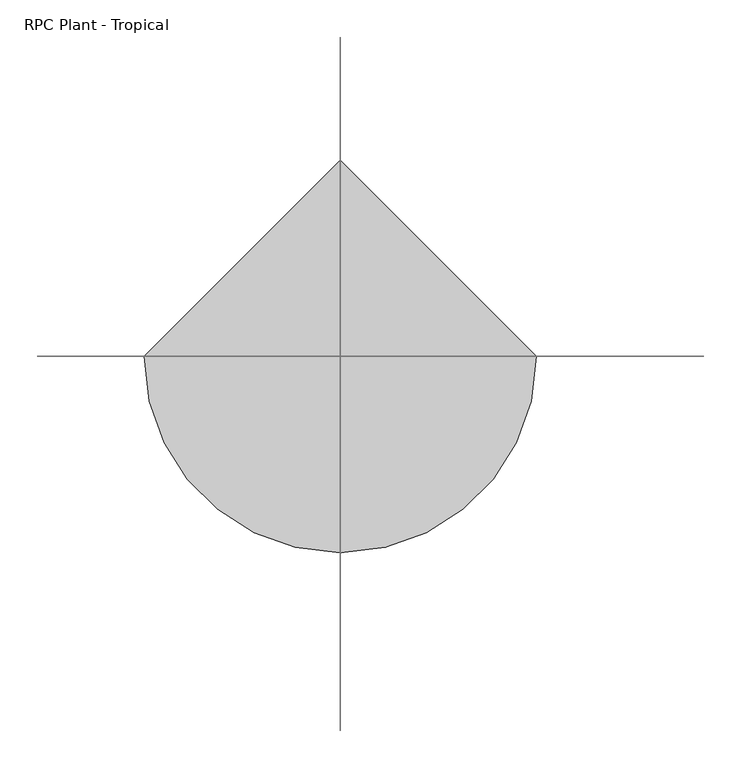
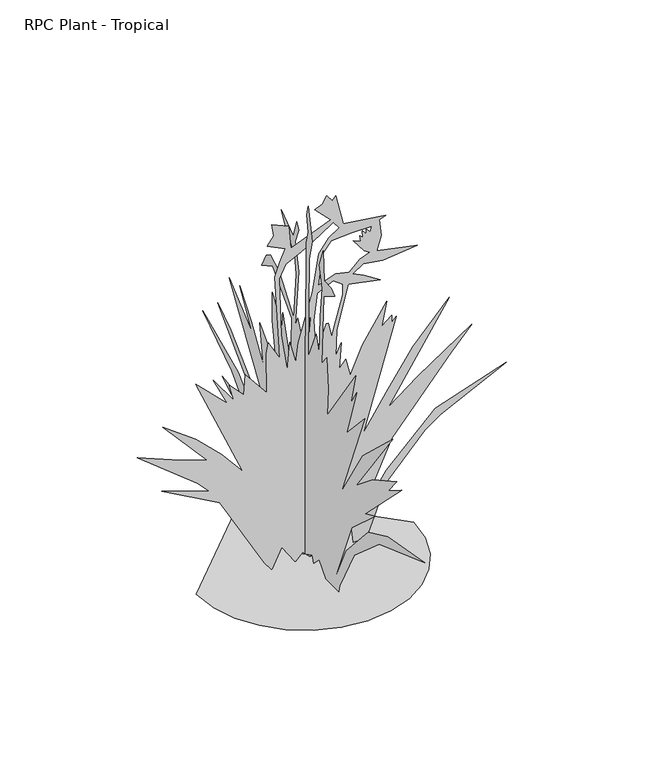
"""IFC4 building model written with IfcOpenShell, lengths in millimetres: geographic element geometry, RPC Plant - Tropical."""

from ifc_helpers import new_model, si_unit, origin, place, context, project, spatial, triangles, source, transform, mapped, element, save


def rpc_plant_tropical_55f6ff97(model_context):
    return source(origin(), model_context, "Body", "Tessellation", [
        triangles([(-264.3380075, 0.0, 0.0272524), (-257.3504617, -60.5688865, 0.0272524), (-237.4475159, -116.1916269, 0.0272524), (-206.2245489, -165.274632, 0.0272524), (-165.274632, -206.2245489, 0.0272524), (-116.1916269, -237.4475159, 0.0272524), (-60.5688865, -257.3504617, 0.0272524), (1.16e-05, -264.3380075, 0.0272524), (60.5688865, -257.3504617, 0.0272524), (116.1916269, -237.4475159, 0.0272524), (165.274632, -206.2245489, 0.0272524), (206.2245489, -165.274632, 0.0272524), (237.4475159, -116.1916269, 0.0272524), (257.3504617, -60.5688865, 0.0272524), (264.3380075, 2.31e-05, 0.0272524), (-3.47e-05, 264.3380075, 0.0272524), (-5.2e-06, -141.3706678, 0.0), (-2.8e-06, -89.4159448, 0.054498), (-3.14e-05, -59.9343958, 33.2735186), (-3.1e-05, -36.3827356, 9.846953), (-3.03e-05, -30.3380374, 26.1345898), (2.2e-06, 22.1351019, 0.0353721), (-2.75e-05, 35.0893666, 22.475361), (-2.7e-05, 50.4325003, 13.9824575), (-2.41e-05, 71.8028075, 80.7852761), (5.2e-06, 91.613049, 0.0211753), (-2.36e-05, 109.0153662, 40.8424698), (-2.42e-05, 112.8357816, 15.9965016), (-1.83e-05, 164.4437961, 134.5614359), (-1.5e-05, 201.3025201, 190.8125718), (-8.6e-06, 314.8967674, 236.0083596), (-6.4e-06, 348.2342674, 257.8737037), (-8.8e-06, 301.5160253, 250.5209003), (-1.18e-05, 246.732487, 231.9590791), (-7.1e-06, 309.0598417, 295.0364789), (8e-07, 430.3017509, 376.6543714), (-7.9e-06, 280.4721063, 309.3519387), (-1.58e-05, 174.5674878, 204.3200503), (-9.8e-06, 240.1660818, 307.4037292), (-3e-07, 367.670363, 434.9626582), (-3.8e-06, 312.5929836, 399.2629114), (-1.14e-05, 210.1351387, 300.3374635), (-1.65e-05, 148.1844779, 220.8381918), (-1.17e-05, 187.1702069, 323.3016323), (3e-07, 320.1596366, 527.8276657), (-6.4e-06, 222.976615, 445.7627257), (-1.5e-06, 274.807899, 534.3072121), (-5.5e-06, 226.7299833, 472.9153562), (-1.02e-05, 175.4651256, 391.7724529), (-6.5e-06, 190.5821898, 491.1144633), (-1.2e-05, 119.3145649, 415.5265626), (-7.8e-06, 137.4532288, 529.6031387), (-5.6e-06, 138.7511692, 601.2540341), (-9.5e-06, 94.9513718, 536.1969586), (-8.4e-06, 93.3989229, 575.3383922), (-1.32e-05, 59.5732078, 463.4487828), (-9.8e-06, 56.2066891, 583.9388483), (-3.7e-06, 136.0049161, 669.1432405), (-2.4e-06, 181.9436545, 644.4467829), (-2.1e-06, 163.9243692, 680.6875214), (-2.5e-06, 147.0399529, 691.5511024), (-4.8e-06, 108.1804607, 671.9067347), (-1e-05, 48.046931, 590.4565101), (-6.9e-06, 36.8709235, 709.0745968), (-5.3e-06, 43.8627887, 753.7100264), (-2e-06, 83.7514831, 804.4440662), (-3e-07, 99.8779606, 836.6538008), (-3.7e-06, 49.136086, 799.8898384), (-2.9e-06, 35.0893666, 845.2923723), (-3.8e-06, 26.4505657, 828.0152292), (-4.3e-06, 41.5678933, 791.3020632), (-7e-06, 26.8495989, 721.233593), (-1.07e-05, 41.5678933, 575.3383922), (-1.05e-05, 30.7698379, 599.0950453), (-1.29e-05, 9.1735731, 551.5843188), (-1.27e-05, -4.2437592, 577.167205), (-5.7e-06, -6.2811965, 815.731822), (-5.1e-06, -13.569935, 847.4513248), (-3.6e-06, -6.9461944, 887.7586756), (-3.1e-06, -14.582304, 914.4007267), (-6.2e-06, -30.3001922, 833.2324253), (-7.2e-06, -17.1413308, 780.7407166), (-1.46e-05, -14.582304, 527.8276657), (-1.38e-05, -46.9765748, 605.5745916), (-1.57e-05, -59.9343958, 560.222854), (-1.28e-05, -63.7807226, 662.0591526), (-1.1e-05, -73.6229771, 738.5157503), (-8.8e-06, -59.9343958, 791.3020632), (-8.5e-06, -68.5729447, 815.05868), (-8.2e-06, -77.2114935, 838.812826), (-1.06e-05, -81.5307611, 763.227396), (-1.2e-05, -110.9300204, 761.8202871), (-1.3e-05, -126.4778813, 751.5510738), (-1.23e-05, -100.3333834, 735.2899298), (-1.17e-05, -79.708316, 722.0590513), (-1.66e-05, -70.7324513, 545.1047725), (-1.68e-05, -92.3897821, 572.3361045), (-1.94e-05, -98.8076044, 495.4324774), (-2.12e-05, -94.4883277, 426.3240867), (-2.14e-05, -213.2677237, 599.0950453), (-2.3e-05, -193.8311193, 517.0301053), (-2.28e-05, -217.5869913, 558.0613217), (-2.48e-05, -176.5542669, 430.6446442), (-2.57e-05, -252.1411685, 512.7095841), (-2.87e-05, -152.798395, 264.3532501), (-2.83e-05, -244.4081376, 413.0424482), (-3.04e-05, -369.3264393, 531.0712541), (-2.98e-05, -215.4274755, 318.343541), (-3.13e-05, -285.475907, 376.1107999), (-3.42e-05, -387.58906, 431.8587779), (-3.39e-05, -351.4829427, 387.4518954), (-3.53e-05, -406.9616784, 422.1127885), (-3.3e-05, -254.1018046, 269.3443517), (-3.43e-05, -295.3336628, 288.109885), (-3.26e-05, -197.6014924, 198.8161167), (-3.48e-05, -118.2442087, 7.3579794), (-3.37e-05, -173.2017281, 125.4509545), (-3.48e-05, -266.8272088, 229.6761334), (-3.73e-05, -347.9879162, 267.302198), (-4.35e-05, -504.8177693, 294.5894314), (-3.69e-05, -312.1281501, 226.3418711), (-3.5e-05, -207.3218293, 133.5593986), (-3.57e-05, -146.3193573, 18.1561127), (117.3305654, 2.31e-05, 0.0405123), (110.3389591, 2.08e-05, 74.4091073), (78.0842327, 2.54e-05, 21.0145808), (55.6151237, 2.49e-05, 46.2313396), (12.5873108, 2.89e-05, 0.0122306), (-5.1707583, 2.92e-05, 18.1490262), (-24.1045425, 3.09e-05, 0.0037426), (-56.6857342, 2.97e-05, 48.3908508), (-81.2114855, 3.28e-05, 0.0181663), (-98.986418, 3.3e-05, 24.1438615), (-207.7917316, 2.63e-05, 216.6390658), (-348.2342674, 2.78e-05, 294.5894314), (-233.774666, 2.51e-05, 255.7146967), (-261.6024369, 2.45e-05, 285.2828592), (-408.7041229, 2.4e-05, 402.5700133), (-324.6782925, 2.24e-05, 368.0386909), (-238.0939517, 2.05e-05, 335.6206115), (-346.0752786, 1.79e-05, 458.719275), (-266.2303157, 1.79e-05, 400.2179767), (-203.8244956, 1.88e-05, 339.715129), (-151.7089902, 2.02e-05, 277.3123428), (-266.1693456, 9.5e-06, 540.784215), (-189.3886398, 1.06e-05, 466.0141786), (-222.976615, 7.9e-06, 536.4662009), (-173.7341084, 9.8e-06, 467.1774796), (-184.1031521, 7.7e-06, 510.5505589), (-149.5492202, 8.4e-06, 473.8373929), (-145.2299525, 5.2e-06, 523.5096517), (-93.3989229, 6.8e-06, 458.719275), (-94.0984351, 9e-07, 559.4354384), (-89.0799006, -9e-07, 586.138496), (-61.0044976, 8e-07, 536.4662009), (-64.4230889, -1.9e-06, 583.7153154), (-73.364658, -1.14e-05, 749.2980864), (-61.7167134, -1.39e-05, 783.3111992), (-47.9079951, -1.63e-05, 813.4864649), (-91.2394163, -1.57e-05, 834.4947756), (-76.5455003, -1.76e-05, 856.3946743), (-80.4413563, -1.92e-05, 886.3260595), (-39.8899707, -2e-05, 869.0464457), (-35.0893666, -1.67e-05, 810.7381588), (62.093907, -2.33e-05, 849.6128935), (23.2207756, -2.39e-05, 888.4850847), (42.4165107, -2.52e-05, 896.5013105), (53.4556125, -2.67e-05, 914.4007267), (66.1944834, -2.63e-05, 896.8848627), (74.7598808, -2.72e-05, 906.7806976), (93.6785752, -2.34e-05, 828.1498867), (196.1872255, -2.7e-05, 813.9157265), (180.8732984, -2.6e-05, 808.5791336), (185.7325766, -2.37e-05, 766.8723043), (174.394515, -2.11e-05, 730.8322803), (273.7385602, -2.41e-05, 709.2371595), (189.3833167, -2e-05, 700.9592491), (142.0676456, -1.83e-05, 708.1576469), (116.0844387, -1.62e-05, 691.9600891), (142.8525086, -1.66e-05, 679.102589), (183.0330503, -1.68e-05, 653.0853544), (105.3178811, -1.44e-05, 669.0848139), (77.0491851, -6.7e-06, 560.5047772), (75.051728, -2.7e-06, 495.4324774), (87.9216592, -5e-06, 524.393573), (83.6900225, -9e-07, 458.719275), (98.8076044, -2.7e-06, 478.1553706), (109.6056554, -5e-07, 432.803633), (138.9439536, -5.8e-06, 499.7708027), (199.0078928, -1.39e-05, 592.0084502), (187.352336, -9.8e-06, 532.1482232), (211.1082079, -1.2e-05, 551.5843188), (211.1082079, -1.1e-05, 534.3072121), (221.9062589, -1.21e-05, 545.1047725), (142.0000807, 7.6e-06, 272.9918035), (197.3987977, 1e-07, 358.912431), (262.4025334, -8.4e-06, 452.8214155), (351.4829427, -1.8e-05, 549.4227502), (202.4694002, 2.3e-06, 318.343541), (273.8909673, -4.1e-06, 372.7275035), (405.4757589, -1.51e-05, 460.8783002), (355.6612487, -9.6e-06, 405.7856601), (211.5270596, 6.8e-06, 235.3906284), (131.6828507, 2.08e-05, 59.5396797), (197.4798247, 1.2e-05, 158.3333043), (317.0659301, -2e-07, 275.0161712), (489.6996878, -1.12e-05, 333.4616226), (330.1571005, 5e-07, 255.2422691), (291.8284444, 3.8e-06, 227.7759587), (199.2240496, 1.38e-05, 127.0808696), (148.478864, 2.13e-05, 0.0507429), (114.3788288, -2.24e-05, 797.4488537), (63.6714996, -2.01e-05, 794.7361559), (42.3199913, -1.75e-05, 767.5631779), (31.8592449, -1.25e-05, 691.9600891), (74.6966352, -1.53e-05, 706.3237473), (107.4461487, -1.62e-05, 698.437092), (132.807564, -1.88e-05, 722.7067589), (157.1176626, -2.05e-05, 732.9912329), (143.9299774, -2.04e-05, 741.276701), (117.5705943, -2.13e-05, 776.2906248), (135.9680906, -2.16e-05, 768.3049204), (133.7021497, -2.24e-05, 783.2401279), (140.693002, -2.24e-05, 777.0983517), (139.840574, -2.33e-05, 793.4610884), (148.478864, -2.3e-05, 782.6634916), (148.8047525, -2.38e-05, 795.162874), (158.4753014, -2.36e-05, 785.4854851), (162.2614257, -2.45e-05, 797.6698431), (36.4967821, -2.03e-05, 819.0008085), (-10.5179706, -1.66e-05, 790.7762959), (-46.6034508, -1.4e-05, 773.6338102), (-62.8378705, -1.14e-05, 741.9143074), (-57.6440741, -2.8e-06, 594.8100597), (-43.7276589, 2.2e-06, 499.7530349), (-37.2488755, -2.2e-06, 568.8613893), (-22.1313685, 5e-07, 512.7095841), (-15.8925131, -2.6e-06, 559.8647), (18.0916476, -1.1e-05, 677.0451565), (33.6138798, -1.74e-05, 772.2038103), (57.6697312, -2.04e-05, 805.3914648), (83.6900225, -2.25e-05, 821.5356829), (68.5729447, -2.3e-05, 840.9743219), (30.2087529, -1.13e-05, 671.65784), (21.8014718, -6.9e-06, 605.0462809), (25.6817059, -2.5e-06, 528.0867342), (30.8554363, -2.8e-06, 528.7344418), (51.5501011, -7.1e-06, 586.290885), (56.0771503, -7.3e-06, 585.6457209), (65.1309854, -5.4e-06, 548.1349654), (69.6580301, -6.8e-06, 568.1831966), (91.6460685, -1.24e-05, 645.7879074), (91.6460685, -1.4e-05, 672.9507116), (68.3644091, -1.4e-05, 690.4106197), (6.9271952, -5.7e-06, 595.3460009), (10.8074288, -4.5e-06, 573.3571904), (13.394269, -6.1e-06, 597.9317079), (15.3343985, -7.9e-06, 627.035055)], [[15, 16, 1], [14, 15, 1], [14, 1, 2], [13, 14, 2], [13, 2, 3], [13, 3, 4], [12, 13, 4], [11, 12, 4], [11, 4, 5], [11, 5, 6], [11, 6, 7], [11, 7, 8], [11, 8, 9], [11, 9, 10], [46, 47, 48], [119, 120, 121], [35, 36, 37], [106, 107, 108], [39, 40, 41], [39, 41, 42], [101, 102, 103], [111, 112, 113], [105, 106, 108], [44, 45, 46], [113, 114, 115], [54, 55, 56], [103, 104, 105], [99, 100, 101], [109, 110, 111], [89, 90, 91], [118, 119, 121], [31, 32, 33], [46, 48, 49], [44, 46, 49], [79, 80, 81], [78, 79, 81], [66, 67, 68], [27, 28, 29], [52, 53, 54], [88, 89, 91], [87, 88, 91], [49, 50, 51], [58, 59, 60], [99, 101, 103], [25, 26, 27], [83, 84, 85], [109, 111, 113], [108, 109, 113], [96, 97, 98], [68, 69, 70], [68, 70, 71], [38, 39, 42], [38, 42, 43], [65, 66, 68], [65, 68, 71], [65, 71, 72], [64, 65, 72], [64, 72, 73], [63, 64, 73], [118, 121, 122], [117, 118, 122], [117, 122, 123], [116, 117, 123], [73, 74, 75], [116, 123, 17], [116, 17, 18], [58, 60, 61], [58, 61, 62], [57, 58, 62], [57, 62, 63], [77, 78, 81], [77, 81, 82], [76, 77, 82], [76, 82, 83], [75, 76, 83], [92, 93, 94], [19, 20, 21], [30, 31, 33], [30, 33, 34], [91, 92, 94], [87, 91, 94], [87, 94, 95], [86, 87, 95], [86, 95, 96], [85, 86, 96], [34, 35, 37], [34, 37, 38], [30, 34, 38], [25, 27, 29], [57, 63, 73], [56, 57, 73], [56, 73, 75], [56, 75, 83], [23, 24, 25], [99, 103, 105], [29, 30, 38], [105, 108, 113], [105, 113, 115], [51, 52, 54], [51, 54, 56], [83, 85, 96], [21, 22, 23], [83, 96, 98], [83, 98, 99], [56, 83, 99], [29, 38, 43], [25, 29, 43], [115, 116, 18], [115, 18, 19], [105, 115, 19], [21, 23, 25], [44, 49, 51], [43, 44, 51], [56, 99, 105], [51, 56, 105], [43, 51, 105], [43, 105, 19], [25, 43, 19], [21, 25, 19], [248, 124, 125], [241, 229, 212], [206, 207, 208], [197, 198, 199], [146, 147, 148], [134, 135, 136], [196, 197, 199], [241, 212, 213], [255, 237, 238], [140, 141, 142], [200, 201, 202], [137, 138, 139], [255, 238, 239], [258, 255, 239], [175, 176, 177], [184, 185, 186], [235, 236, 237], [180, 181, 182], [189, 190, 191], [144, 145, 146], [140, 142, 143], [247, 248, 125], [171, 172, 173], [200, 202, 203], [199, 200, 203], [193, 194, 195], [237, 255, 256], [220, 221, 222], [148, 149, 150], [137, 139, 140], [224, 225, 226], [229, 241, 242], [195, 196, 199], [222, 223, 224], [153, 154, 155], [179, 180, 182], [150, 151, 152], [226, 227, 228], [191, 192, 193], [186, 187, 188], [169, 170, 171], [175, 177, 178], [152, 153, 155], [195, 199, 203], [161, 162, 163], [240, 241, 213], [240, 213, 214], [165, 166, 167], [167, 168, 169], [165, 167, 169], [165, 169, 171], [191, 193, 195], [189, 191, 195], [188, 189, 195], [239, 240, 214], [239, 214, 215], [125, 126, 127], [124, 248, 249], [124, 249, 250], [161, 163, 164], [160, 161, 164], [159, 160, 164], [131, 132, 133], [144, 146, 148], [129, 130, 131], [131, 133, 134], [206, 208, 209], [205, 206, 209], [205, 209, 210], [204, 205, 210], [204, 210, 211], [204, 211, 124], [204, 124, 250], [246, 247, 125], [195, 203, 204], [144, 148, 150], [144, 150, 152], [158, 159, 164], [127, 128, 129], [246, 125, 127], [246, 127, 129], [246, 129, 131], [136, 137, 140], [136, 140, 143], [136, 143, 144], [134, 136, 144], [131, 134, 144], [220, 222, 224], [220, 224, 226], [220, 226, 228], [219, 220, 228], [131, 144, 152], [258, 239, 215], [174, 175, 178], [186, 188, 195], [215, 216, 217], [131, 152, 155], [157, 158, 164], [217, 218, 219], [186, 195, 204], [219, 228, 229], [245, 246, 131], [245, 131, 215], [244, 245, 215], [254, 244, 215], [254, 215, 217], [253, 254, 217], [252, 253, 217], [257, 258, 215], [184, 186, 204], [184, 204, 250], [183, 184, 250], [183, 250, 251], [182, 183, 251], [182, 251, 252], [182, 252, 217], [179, 182, 217], [179, 217, 219], [178, 179, 219], [174, 178, 219], [174, 219, 229], [173, 174, 229], [171, 173, 229], [171, 229, 242], [165, 171, 242], [165, 242, 243], [165, 243, 230], [164, 165, 230], [164, 230, 231], [164, 231, 232], [157, 164, 232], [157, 232, 233], [156, 157, 233], [156, 233, 234], [156, 234, 235], [155, 156, 235], [131, 155, 235], [131, 235, 237], [131, 237, 256], [215, 131, 256], [257, 215, 256]], closed=False),
    ])


if __name__ == "__main__":
    model = new_model("IFC4")
    model_context = context("Model", 3, world=origin())
    ifc_project = project(units=[si_unit("LENGTHUNIT", "METRE", prefix="MILLI")], contexts=[model_context])
    site = spatial("IfcSite", under=ifc_project)
    building = spatial("IfcBuilding", under=site)
    placement = place(None, origin())
    rpc_plant_tropical_shape = rpc_plant_tropical_55f6ff97(model_context)
    element("IfcGeographicElement", 1, ObjectType="RPC Plant - Tropical", at=placement, inside=building, context=model_context, shape_type="MappedRepresentation", body=[
        mapped(rpc_plant_tropical_shape, transform((0.0, 0.0, 0.0), x_axis=(1.0, 0.0, 0.0), y_axis=(0.0, 1.0, 0.0), z_axis=(0.0, 0.0, 1.0))),
    ])
    save(model, "model.ifc")

# Revit data of these elements
# Type "RPC Plant - Tropical"
#   built-in parameter 1005198 = "{2, 15},{39, RPC-16-FWM5-GM7X-C67P-4000-ST1L-LVER-AU},{1, 0},{1, 0},{2, 35},{1, 8},{5, Color},{1, 0},{1, 0},{3, 0.8},{3, 0.8},{3, 0.8},{1, 8},{7, BBoxMin},{1, 0},{1, 0},{1, 0},{1, 0},{1, 0},{1, 8},{7, BBoxMax},{1, 0},{1, 0},{1, 0},{1, 0},{1, 0},{2, 11},{9, RPCTypeId},{1, 0},{1, 0},{39, RPC-16-FWM5-GM7X-C67P-4000-ST1L-LVER-AU},{1, 6},{14, RPCPlantHeight},{1, 0},{1, 0},{1, 3},{2, 11},{7, keyword},{1, 0},{1, 0},{99, :Geometry:RPC:Crane Lily:strelitzia:reinae:crane lily:plants:shrub:flower:tropical:bird-of-paradise},{2, 11},{8, category},{1, 0},{1, 0},{17, :Shrubs [General]},{2, 11},{12, LocalizedUID},{1, 0},{1, 0},{10, Crane Lily},{2, 14},{6, Height},{1, 0},{1, 0},{1, 3},{1, 2},{16, Cast Reflections},{1, 0},{1, 0},{1, 0},{1, 2},{12, Cast Shadows},{1, 0},{1, 0},{1, 1},{1, 2},{9, Lock View},{1, 0},{1, 0},{1, 0},{1, 4},{5, ViewC},{1, 0},{1, 0},{1, 0},{2, 11},{20, AdvancedUIDefinition},{1, 0},{1, 0},{0, },{2, 11},{10, AssetLibID},{1, 0},{1, 0},{36, 4D3F6E72-3F99-4203-98E9-AF80B3C7A7A4},{2, 11},{10, BaseSchema},{1, 0},{1, 0},{9, RPCSchema},{2, 11},{12, ExchangeGUID},{1, 0},{1, 0},{0, },{1, 2},{6, Hidden},{1, 0},{1, 0},{1, 0},{1, 4},{11, RPCCategory},{1, 0},{1, 0},{1, 0},{2, 11},{8, RPCImage},{1, 0},{1, 0},{0, },{1, 4},{13, SchemaVersion},{1, 0},{1, 0},{1, 4},{2, 11},{12, UIDefinition},{1, 0},{1, 0},{0, },{2, 11},{6, UIName},{1, 0},{1, 0},{39, RPC-16-FWM5-GM7X-C67P-4000-ST1L-LVER-AU},{2, 11},{11, VersionGUID},{1, 0},{1, 0},{9, RPCSchema},{2, 11},{9, assettype},{1, 0},{1, 0},{11, RPCGeometry},{2, 11},{11, description},{1, 0},{1, 0},{0, },{2, 11},{9, localname},{1, 0},{1, 0},{3, RPC},{2, 11},{9, localtype},{1, 0},{1, 0},{3, RPC},{1, 4},{8, revision},{1, 0},{1, 0},{1, 1},{2, 11},{9, thumbnail},{1, 0},{1, 0},{0, },{1, 4},{7, version},{1, 0},{1, 0},{1, 1},{1, 2},{20, RPC_Cast Reflections},{1, 0},{1, 0},{1, 1},{1, 2},{16, RPC_Cast Shadows},{1, 0},{1, 0},{1, 1},{1, 2},{13, RPC_Lock View},{1, 0},{1, 0},{1, 0},{1, 4},{9, RPC_ViewC},{1, 0},{1, 0},{1, 0},{21, assetlibrary_base.fbx},{1, 5},"
#   built-in parameter 1005195 = "RPC-16-FWM5-GM7X-C67P-4000-ST1L-LVER-AU"
#   Assembly Code = "G2050500"
#   Height = 3' - 0"
#   Default Elevation = 0
